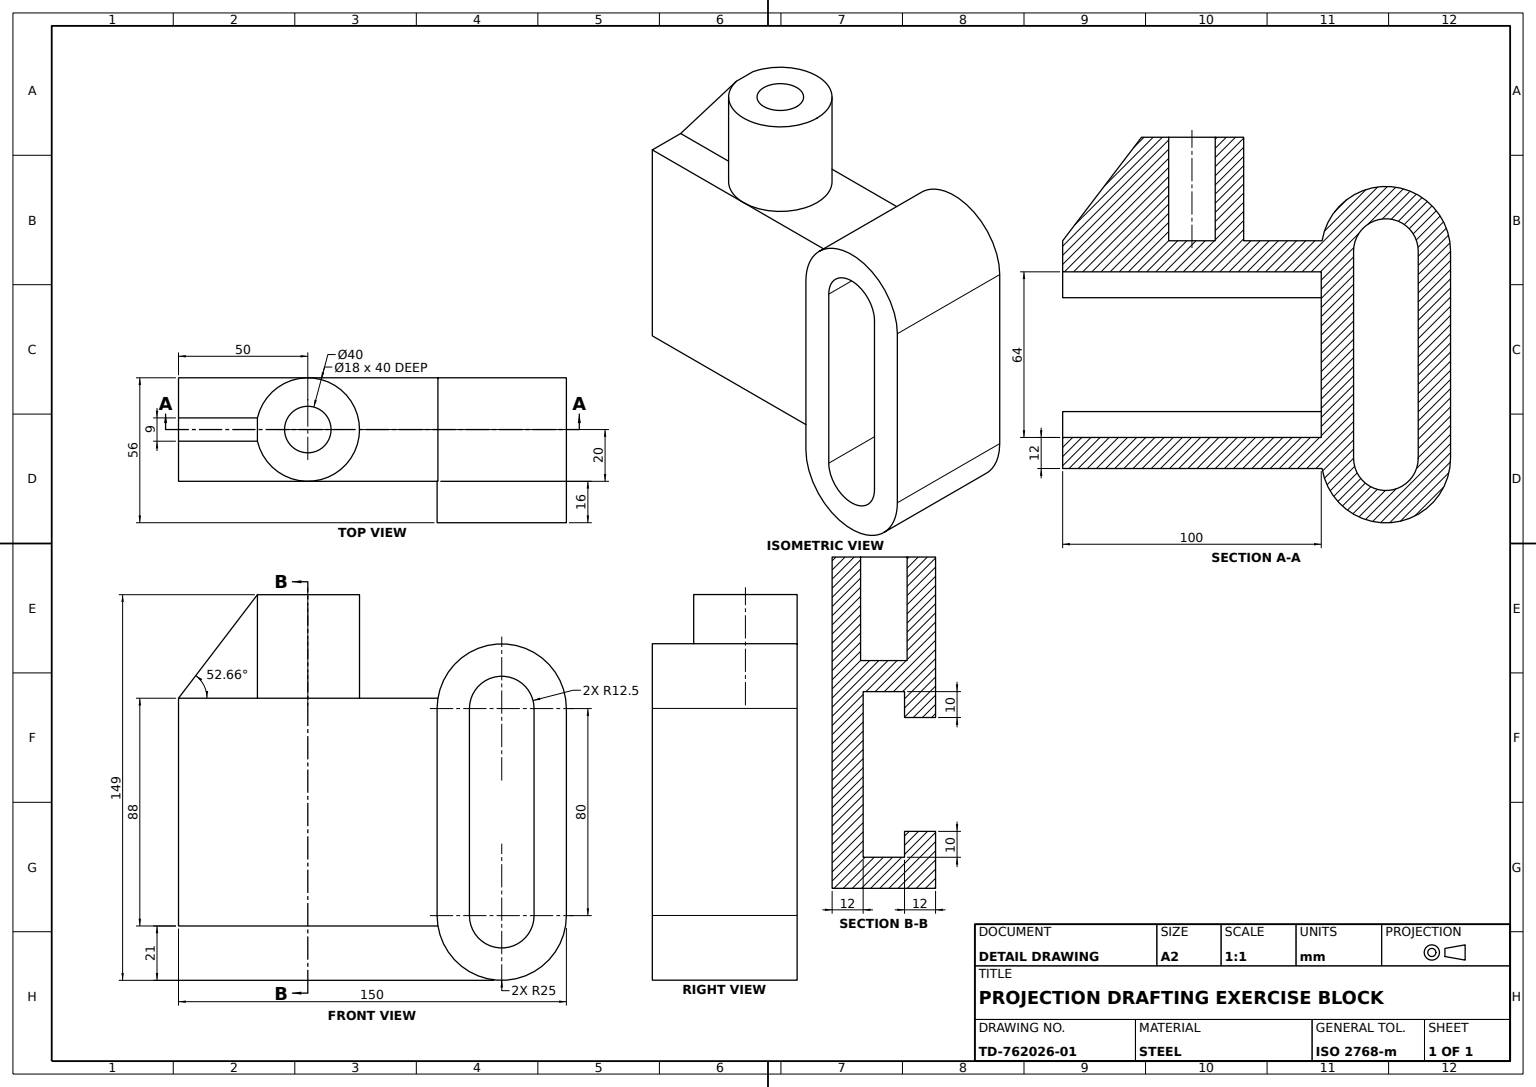
SolidWorks part; units mm, degrees
material "Plain Carbon Steel"
ref_plane "Front Plane" through (0, 0, 0) normal (0, 0, 1) x (1, 0, 0)
ref_plane "Top Plane" through (0, 0, 0) normal (0, 1, 0) x (1, 0, 0)
ref_plane "Right Plane" through (0, 0, 0) normal (1, 0, 0) x (0, 0, -1)
sketch "Base Block Sketch" plane through (0, 0, 0) normal (0, 0, 1) x (1, 0, 0)
  line L1 (-20, -44) -> (20, -44)
  line L2 (-20, -44) -> (-20, 44)
  line L3 (-20, 44) -> (20, 44)
  line L4 (20, -44) -> (20, 44)
  line L5 (-20, -44) -> (20, 44) construction
  line L6 (-20, 44) -> (20, -44) construction
  point P0 (0, 0)
  dimension "D1" = 40
  dimension "D2" = 88
extrude "Base Block" add sketch "Base Block Sketch" along normal mid plane 100
sketch "C-Channel Cut Sketch" plane through (0, 0, 50) normal (0, 0, 1) x (1, 0, 0)
  line L0 (-20, 22) -> (-8, 22)
  line L1 (-8, 22) -> (-8, 32)
  line L2 (-8, 32) -> (8, 32)
  line L3 (8, 32) -> (8, -32)
  line L4 (20, -44) -> (20, 44)
  line L5 (20, 44) -> (-20, 44)
  line L6 (-20, 44) -> (-20, -44)
  line L7 (-20, -44) -> (20, -44)
  line L10 (-20, 22) -> (-20, -22)
  line L12 (8, -32) -> (-8, -32)
  line L13 (-8, -32) -> (-8, -22)
  line L14 (-8, -22) -> (-20, -22)
  line L15 (-63.214, 0) -> (53.9863, 0) construction
  line L16 (20, -44) -> (20, 44) construction
  line L19 (20, 44) -> (-20, 44) construction
  dimension "D2" = 12
  dimension "D3" = 22
  dimension "D6" = 12
  dimension "D7" = 64
  dimension "D1" = 0
extrude "C-Channel Cut" cut sketch "C-Channel Cut Sketch" against normal through all
sketch "Slotted Lug Sketch" plane through (20, 0, 0) normal (1, 0, 0) x (0, 0, -1)
  line L0 (0, 0) -> (106.2979, 0) construction
  line L1 (75, 44) -> (75, -44) construction
  line L2 (100, 40) -> (100, -40)
  line L3 (62.5, 40) -> (62.5, -40)
  line L4 (50, -44) -> (50, 44)
  line L5 (50, 44) -> (-50, 44)
  line L6 (-50, 44) -> (-50, -44)
  line L7 (-50, -44) -> (50, -44)
  line L8 (50, -44) -> (50, 44)
  line L12 (87.5, 40) -> (87.5, -40)
  arc A0 (100, 40) -> (50, 40) centre (75, 40) ccw
  arc A1 (87.5, 40) -> (62.5, 40) centre (75, 40) ccw
  arc A2 (100, -40) -> (50, -40) centre (75, -40) cw
  arc A3 (87.5, -40) -> (62.5, -40) centre (75, -40) cw
  dimension "D4" = 50
  dimension "D5" = 25
  dimension "D2" = 25
  dimension "D3" = 4
  dimension "D1" = 0
extrude "Slotted Lug" add sketch "Slotted Lug Sketch" against normal through all contours A2 L2 A0 L8 L12 A3 L3 A1
sketch "Lug Rim Sketch" plane through (20, 0, 0) normal (1, 0, 0) x (0, 0, -1)
  line L0 (87.5, 40) -> (87.5, -40) construction
  line L1 (62.5, 40) -> (62.5, -40) construction
  line L2 (87.5, 40) -> (87.5, -40)
  line L3 (62.5, 40) -> (62.5, -40)
  line L4 (50, 40) -> (50, -40)
  line L6 (50, -44) -> (50, -40)
  line L7 (100, -40) -> (100, 40)
  line L8 (50, 40) -> (50, 44)
  line L9 (50, 44) -> (-50, 44)
  line L10 (-50, 44) -> (-50, -44)
  line L11 (-50, -44) -> (50, -44)
  line L12 (50, -44) -> (50, -40)
  line L13 (100, -40) -> (100, 40)
  line L14 (50, 40) -> (50, 44)
  arc A0 (62.5, -40) -> (87.5, -40) centre (75, -40) ccw construction
  arc A1 (87.5, 40) -> (62.5, 40) centre (75, 40) ccw construction
  arc A2 (50, -40) -> (100, -40) centre (75, -40) ccw
  arc A3 (100, 40) -> (50, 40) centre (75, 40) ccw
  arc A4 (50, -40) -> (100, -40) centre (75, -40) ccw
  arc A5 (100, 40) -> (50, 40) centre (75, 40) ccw
  arc A6 (62.5, -40) -> (87.5, -40) centre (75, -40) ccw
  arc A7 (87.5, 40) -> (62.5, 40) centre (75, 40) ccw
  arc M10 (50, -40) -> (100, -40) centre (75, -40) ccw
  line M11 (100, -40) -> (100, 40)
  arc M12 (100, 40) -> (50, 40) centre (75, 40) ccw
  line M17 (87.5, 40) -> (87.5, -40)
  arc M18 (87.5, -40) -> (62.5, -40) centre (75, -40) cw
  line M19 (62.5, -40) -> (62.5, 40)
  arc M20 (62.5, 40) -> (87.5, 40) centre (75, 40) cw
  dimension "D1" = 0
extrude "Lug Rim" add sketch "Lug Rim Sketch" along normal blind 16 contours L4 M12 M10 M11 M20 M17 M18 M19
sketch "Boss Cylinder Sketch Ø18" plane through (0, 44, 0) normal (0, 1, 0) x (1, 0, 0)
  circle A0 centre (0, 0) radius 20
  circle A1 centre (0, 0) radius 9
  dimension "D1" = 40
  dimension "D2" = 18
extrude "Boss Cylinder Ø18" add sketch "Boss Cylinder Sketch Ø18" along normal blind 40
sketch "Boss Extension Sketch" plane through (0, 44, 0) normal (0, 1, 0) x (1, 0, 0)
  line L0 (20, -50) -> (-20, -50) construction
  line L2 (-4.5, -19.4872) -> (-4.5, -50)
  line L3 (-4.5, -50) -> (4.5, -50)
  line L4 (4.5, -19.4872) -> (4.5, -50)
  line L5 (0, 32.6055) -> (0, -53.7358) construction
  arc A0 (-20, 0) -> (20, 0) centre (0, 0) ccw construction
  arc A1 (-4.5, -19.4872) -> (4.5, -19.4872) centre (0, 0) ccw
  dimension "D1" = 9
extrude "Boss Extension" add sketch "Boss Extension Sketch" along normal blind 40
sketch "Boss Bore Sketch" plane through (-4.5, 0, 0) normal (-1, 0, 0) x (0, 0, 1)
  line L0 (19.4872, 84) -> (50, 44)
  line L4 (19.4872, 44) -> (50, 44)
  line L5 (50, 44) -> (50, 84)
  line L6 (50, 84) -> (19.4872, 84)
  line L7 (19.4872, 84) -> (19.4872, 44)
  line L9 (50, 44) -> (50, 84)
  line L10 (50, 84) -> (19.4872, 84)
  dimension "D1" = 0
extrude "Boss Bore Cut" cut sketch "Boss Bore Sketch" against normal blind 40
sketch "Gusset Rib A Sketch" plane through (0, 0, -50) normal (0, 0, -1) x (-1, 0, 0)
  line L4 (-20, 40) -> (20, 40)
  line L5 (20, 40) -> (20, 44)
  line L6 (20, 44) -> (-20, 44)
  line L7 (-20, 44) -> (-20, 40)
  line L8 (-20, 40) -> (20, 40)
  line L9 (20, 40) -> (20, 44)
  line L10 (20, 44) -> (-20, 44)
  line L11 (-20, 44) -> (-20, 40)
  dimension "D1" = 0
extrude "Gusset Rib A" add sketch "Gusset Rib A Sketch" along normal blind 10
sketch "Gusset Rib B Sketch" plane through (0, 0, -50) normal (0, 0, -1) x (-1, 0, 0)
  line L4 (20, -40) -> (-20, -40)
  line L5 (-20, -40) -> (-20, -44)
  line L6 (-20, -44) -> (20, -44)
  line L7 (20, -44) -> (20, -40)
  line L8 (20, -40) -> (-20, -40)
  line L9 (-20, -40) -> (-20, -44)
  line L10 (-20, -44) -> (20, -44)
  line L11 (20, -44) -> (20, -40)
  dimension "D1" = 0
extrude "Gusset Rib B" add sketch "Gusset Rib B Sketch" along normal blind 10
